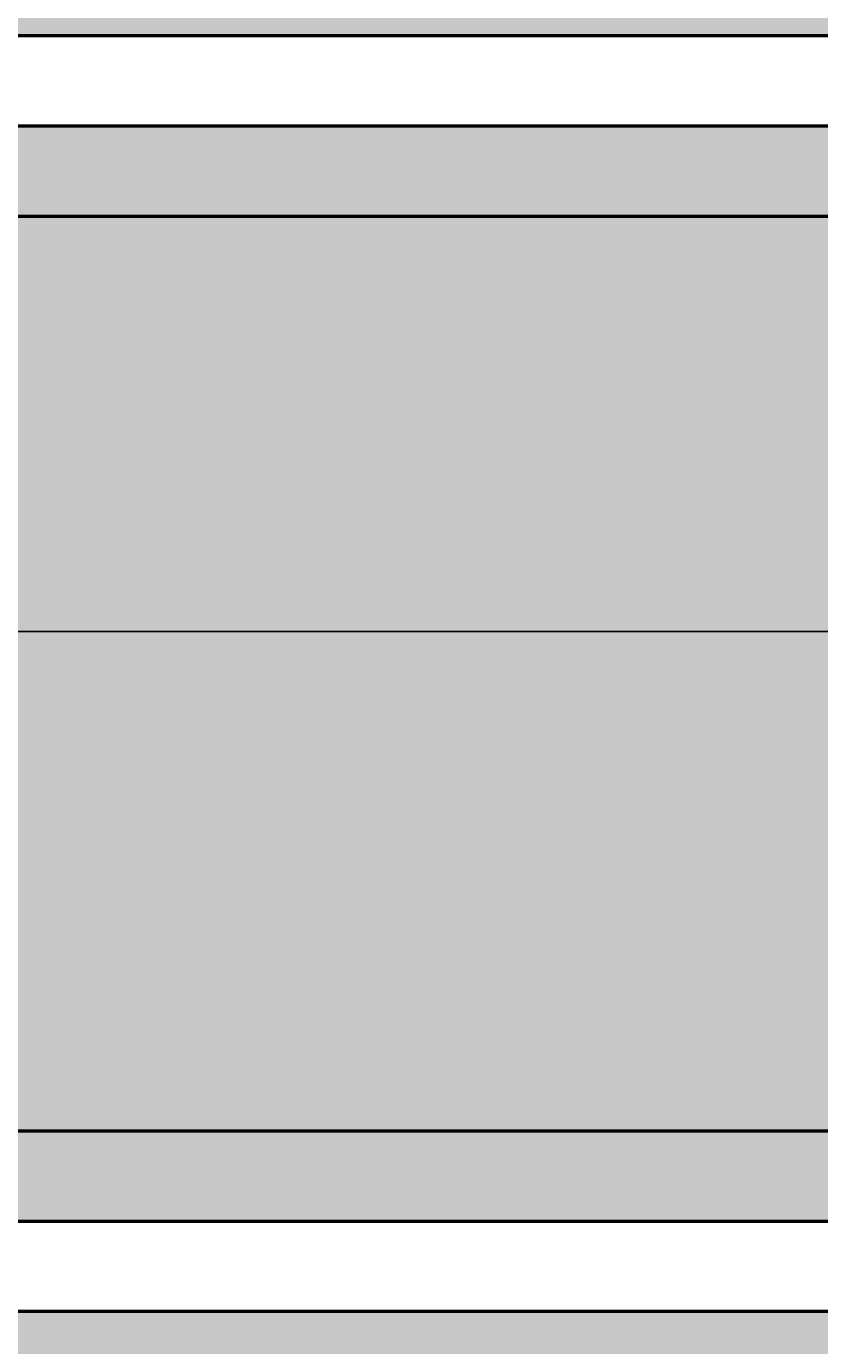
# Model space of a CAD drawing. Units: inches. Extents: x -12 to 334, y -10 to 186.
# Tile 18 of 77: x 88 to 106, y 65 to 94. Entities that reach past the tile are written whole.
import ezdxf

# ---------------------------------------------------------------- set-up
doc = ezdxf.new("R2010")
doc.units = ezdxf.units.IN
doc.header["$MEASUREMENT"] = 0
for name, color, linetype, lineweight in [('M-DIMS', 2, 'Continuous', 18), ('M-EQPM', 7, 'Continuous', 50), ('M-EQPM-PATT', 8, 'Continuous', 18)]:
    doc.layers.add(name, color=color, linetype=linetype, lineweight=lineweight)
doc.styles.get("Standard").update_dxf_attribs({"font": 'arial.ttf'})
doc.dimstyles.get("Standard").update_dxf_attribs({"dimtxt": 0.18, "dimasz": 0.18, "dimexe": 0.18, "dimexo": 0.0625, "dimgap": 0.09, "dimtad": 0, "dimtih": 1, "dimtoh": 1, "dimdec": 4, "dimzin": 0, "dimdsep": 46, "dimtxsty": 'Standard', "dimcen": 0.09, "dimadec": 0, "dimazin": 0, "dimtfac": 1, "dimtdec": 4, "dimtofl": 0, "dimtmove": 0, "dimatfit": 3, "dimfxl": 1, "dimtolj": 1, "dimtzin": 0, "dimarcsym": 0})

# ---------------------------------------------------------------- blocks, each defined once
blk = doc.blocks.new('*D1')
at = {"layer": 'Defpoints', "color": 0, "transparency": 16777216}
for p in [(281.426, 91.899), (3.376, 80.692), (281.426, 14.304)]:
    blk.add_point(p, dxfattribs=at)
at = {"layer": 'M-DIMS', "color": 0, "lineweight": -2, "transparency": 16777216}
for p, q in [((281.426, 91.836), (281.426, 14.124)), ((3.376, 80.629), (3.376, 14.124)), ((3.556, 14.304), (141.935, 14.304)), ((281.246, 14.304), (142.867, 14.304))]:
    blk.add_line(p, q, dxfattribs=at)
at = {"layer": 'M-DIMS', "color": 0, "transparency": 16777216}
for points in [[(3.556, 14.334), (3.556, 14.274), (3.376, 14.304)], [(281.246, 14.334), (281.246, 14.274), (281.426, 14.304)]]:
    blk.add_solid(points, dxfattribs=at)
at = {"layer": 'M-DIMS', "color": 0, "transparency": 16777216, "insert": (142.401, 14.304), "char_height": 0.18, "attachment_point": 5}
blk.add_mtext('\\A1;278.05', dxfattribs=at)
blk = doc.blocks.new('*D35')
at = {"layer": 'Defpoints', "color": 0, "transparency": 16777216}
for p in [(216.428, 98.108), (-11.174, 61.105), (216.428, 61.105)]:
    blk.add_point(p, dxfattribs=at)
at = {"layer": 'M-DIMS', "color": 0, "lineweight": -2, "transparency": 16777216}
for p, q in [((216.365, 98.108), (-11.354, 98.108)), ((-11.174, 97.928), (-11.174, 79.788)), ((-11.174, 61.285), (-11.174, 79.424)), ((216.365, 61.105), (-11.354, 61.105))]:
    blk.add_line(p, q, dxfattribs=at)
at = {"layer": 'M-DIMS', "color": 0, "transparency": 16777216}
for points in [[(-11.204, 97.928), (-11.144, 97.928), (-11.174, 98.108)], [(-11.204, 61.285), (-11.144, 61.285), (-11.174, 61.105)]]:
    blk.add_solid(points, dxfattribs=at)
at = {"layer": 'M-DIMS', "color": 0, "transparency": 16777216, "insert": (-11.174, 79.606), "char_height": 0.18, "attachment_point": 5}
blk.add_mtext('\\A1;37', dxfattribs=at)
blk = doc.blocks.new('*D39')
at = {"layer": 'Defpoints', "color": 0, "transparency": 16777216}
for p in [(279.726, 80.692), (-11.174, 45.854), (269.381, 45.854)]:
    blk.add_point(p, dxfattribs=at)
at = {"layer": 'M-DIMS', "color": 0, "lineweight": -2, "transparency": 16777216}
for p, q in [((279.664, 80.692), (-11.354, 80.692)), ((-11.174, 80.512), (-11.174, 63.455)), ((-11.174, 46.034), (-11.174, 63.091)), ((269.318, 45.854), (-11.354, 45.854))]:
    blk.add_line(p, q, dxfattribs=at)
at = {"layer": 'M-DIMS', "color": 0, "transparency": 16777216}
for points in [[(-11.204, 80.512), (-11.144, 80.512), (-11.174, 80.692)], [(-11.204, 46.034), (-11.144, 46.034), (-11.174, 45.854)]]:
    blk.add_solid(points, dxfattribs=at)
at = {"layer": 'M-DIMS', "color": 0, "transparency": 16777216, "insert": (-11.174, 63.273), "char_height": 0.18, "attachment_point": 5}
blk.add_mtext('\\A1;34.84', dxfattribs=at)

msp = doc.modelspace()

# ---------------------------------------------------------------- hatches: boundary and pattern name
at = {"layer": 'M-EQPM-PATT'}
h = msp.add_hatch(color=256, dxfattribs=at)
h.set_gradient(color1=(205, 32, 39), color2=(205, 32, 39), tint=1)
h.paths.add_polyline_path([(64.5, 80.754), (64.5, 89.8963), (226.6083, 89.8963, -1), (226.6083, 69.6117), (64.5, 69.6117), (64.5, 78.754), (4.4744, 78.754, 0.384914), (23.5807, 61.4872), (37.1002, 61.4872), (37.1002, 33.6752), (53.1002, 33.6752), (53.1002, 61.4872), (64.5, 61.4872), (64.5, 63.6117), (226.6083, 63.6117, 1), (226.6083, 95.8963), (64.5, 95.8963), (64.5, 99.8958), (53.1002, 99.8958), (53.1002, 127.7078), (37.1002, 127.7078), (37.1002, 99.8958), (23.5807, 99.8958, 0.4132606), (4.3766, 80.754)])
h.paths.add_polyline_path([(64.5, 91.8963), (64.5, 93.8963), (226.6083, 93.8963, -1), (226.6083, 65.6117), (64.5, 65.6117), (64.5, 67.6117), (226.6083, 67.6117, 1), (226.6083, 91.8963)], flags=16)
h = msp.add_hatch(color=256, dxfattribs=at)
h.set_gradient(color1=(94, 103, 175), color2=(94, 103, 175), tint=1)
h.paths.add_polyline_path([(129.093, 89.8963), (86.8879, 89.8963), (86.8879, 69.6117), (129.093, 69.6117)], flags=17)
h.paths.add_polyline_path([(170.9079, 89.8963), (130.8573, 89.8963), (130.8573, 69.6117), (170.9079, 69.6117)], flags=17)
h.paths.add_polyline_path([(216.4278, 89.8963), (172.6722, 89.8963), (172.6722, 69.6117), (216.4278, 69.6117)], flags=17)
h.paths.add_polyline_path([(245.9354, 82.6969), (247.9354, 82.6969), (247.9354, 46.8541), (268.3808, 46.8541, 0.0998398), (279.7263, 80.6915), (251.9801, 80.6915, 0.4142136), (231.7758, 100.8958), (84.7229, 100.8958), (84.7229, 109.0583), (83.7229, 109.0583), (83.7229, 95.8963), (129.093, 95.8963), (129.093, 98.1081), (130.8573, 98.1081), (130.8573, 95.8963), (170.9079, 95.8963), (170.9079, 98.1081), (172.6722, 98.1081), (172.6722, 95.8963), (216.4278, 95.8963), (216.4278, 98.1081), (218.1922, 98.1081), (218.1922, 95.8963), (226.6083, 95.8963, -1), (226.6083, 63.6117), (218.1922, 63.6117), (218.1922, 61.1045), (216.4278, 61.1045), (216.4278, 63.6117), (172.6722, 63.6117), (172.6722, 61.1045), (170.9079, 61.1045), (170.9079, 63.6117), (130.8573, 63.6117), (130.8573, 61.1045), (129.093, 61.1045), (129.093, 63.6117), (87.8879, 63.6117), (87.8879, 56.3205), (105.8919, 56.3205), (105.8919, 28.8541), (115.8919, 28.8541), (115.8919, 46.8541), (222.5761, 46.8541), (222.5761, 30.8541), (232.5761, 30.8541), (232.5761, 46.8541), (245.9354, 46.8541)])
h.paths.add_polyline_path([(86.8879, 89.8963), (75.9244, 89.8963), (75.9244, 69.6117), (86.8879, 69.6117)])
h.paths.add_polyline_path([(83.7229, 109.0583), (75.9244, 109.0583), (75.9244, 95.8963), (83.7229, 95.8963)])
h.paths.add_polyline_path([(226.6083, 89.8963), (218.1922, 89.8963), (218.1922, 69.6117), (226.6083, 69.6117, 1)], flags=17)

# ---------------------------------------------------------------- linework, layer by layer
at = {"layer": 'M-EQPM'}
for points in [[(64.5, 65.6117), (226.6083, 65.6117, 1), (226.6083, 93.8963), (64.5, 93.8963)], [(64.5, 67.6117), (226.6083, 67.6117, 1), (226.6083, 91.8963), (64.5, 91.8963)], [(64.5, 69.6117), (226.6083, 69.6117, 1), (226.6083, 89.8963), (64.5, 89.8963)]]:
    msp.add_lwpolyline(points, format="xyb", dxfattribs=at)

# ---------------------------------------------------------------- dimensions: what is measured, and where the dimension line sits
at = {"layer": 'M-DIMS'}
for base, p1, p2, override, picture, middle in [((-11.1736, 61.1045), (216.4278, 98.1081), (216.4278, 61.1045), {"dimdec": 0, "dimlfac": 1, "dimrnd": 0, "dimzin": 0, "dimdsep": 46, "dimlunit": 2}, '*D35', (-11.1735, 79.6063)), ((-11.1736, 45.8541), (279.7263, 80.6915), (269.3808, 45.8541), {"dimdec": 2, "dimlfac": 1, "dimrnd": 0, "dimzin": 0, "dimdsep": 46, "dimlunit": 2}, '*D39', (-11.1735, 63.2728))]:
    dim = msp.add_linear_dim(base=base, p1=p1, p2=p2, angle=90, dimstyle='Standard', override=override, dxfattribs=at)
    dim.commit()
    dim.dimension.update_dxf_attribs({"geometry": picture, "text_midpoint": middle})
dim = msp.add_linear_dim(base=(281.4256, 14.3041), p1=(3.3765, 80.6915), p2=(281.4256, 91.8988), dimstyle='Standard', override={"dimdec": 2, "dimlfac": 1, "dimrnd": 0, "dimzin": 0, "dimdsep": 46, "dimlunit": 2}, dxfattribs=at)
dim.commit()
dim.dimension.update_dxf_attribs({"geometry": '*D1', "text_midpoint": (142.401, 14.3041)})

doc.saveas('drawing.dxf')
